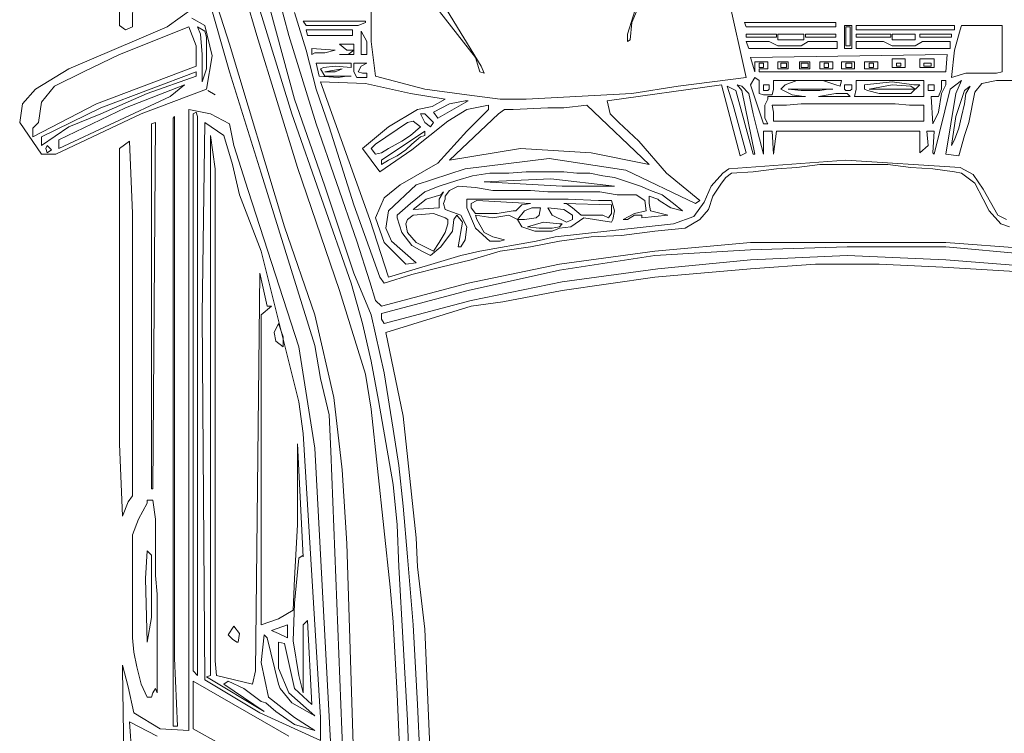
# Model space of a CAD drawing. Units: inches. Extents: x -36302355 to 648, y -221479757 to 75.
# Tile 7 of 37: x 182 to 209, y -484 to -465. Entities that reach past the tile are written whole.
import ezdxf

# ---------------------------------------------------------------- set-up
doc = ezdxf.new("R2010")
doc.units = ezdxf.units.IN
doc.header["$MEASUREMENT"] = 0
doc.layers.add('A-EQPM-VEHC', color=8, linetype='Continuous', lineweight=13)

msp = doc.modelspace()

# ---------------------------------------------------------------- linework, layer by layer
at = {"layer": 'A-EQPM-VEHC'}
for p, q in [((185.107, -459.219), (185.107, -465.157)), ((202.134, -466.571), (201.032, -461.617)), ((185.461, -465.195), (185.5, -462.049)), ((188.842, -465.431), (187.821, -461.932)), ((188.96, -462.6), (189.708, -465.431)), ((191.95, -463.307), (191.95, -465.588)), ((199.736, -463.386), (199.027, -465.078)), ((188.567, -463.583), (189.786, -467.555)), ((198.909, -465.392), (199.46, -463.662)), ((187.467, -464.213), (188.095, -466.415)), ((187.623, -464.172), (188.095, -465.667)), ((187.112, -464.685), (186.405, -465.195)), ((189.865, -467.162), (189.197, -464.723)), ((189.865, -464.802), (190.18, -465.825)), ((193.64, -464.565), (194.78, -466.022)), ((194.938, -466.257), (193.994, -464.723)), ((187.426, -465.157), (187.074, -464.96)), ((190.101, -465.037), (191.792, -465.037)), ((190.18, -465.157), (190.101, -465.037)), ((191.792, -465.037), (191.792, -465.078)), ((185.107, -465.157), (185.265, -465.274)), ((186.995, -465.195), (185.107, -465.943)), ((185.265, -465.274), (185.461, -465.195)), ((186.405, -465.195), (185.579, -465.55)), ((187.191, -465.706), (186.995, -465.195)), ((187.426, -465.313), (187.23, -465.195)), ((187.23, -465.195), (187.309, -465.392)), ((187.623, -465.981), (187.426, -465.157)), ((187.467, -465.471), (187.426, -465.313)), ((191.596, -465.157), (190.18, -465.157)), ((190.18, -465.274), (191.438, -465.274)), ((190.22, -465.431), (190.18, -465.274)), ((191.438, -465.274), (191.438, -465.431)), ((191.792, -465.078), (191.596, -465.157)), ((191.831, -465.588), (191.674, -465.313)), ((191.674, -465.313), (191.674, -465.943)), ((199.027, -465.078), (198.988, -465.55)), ((204.572, -465.078), (202.094, -465.078)), ((202.094, -465.078), (202.134, -465.195)), ((202.134, -465.195), (204.572, -465.195)), ((204.572, -465.195), (204.572, -465.078)), ((205.005, -465.157), (204.808, -465.157)), ((204.808, -465.157), (204.808, -465.785)), ((204.965, -465.195), (204.847, -465.195)), ((204.847, -465.195), (204.847, -465.706)), ((204.965, -465.706), (204.965, -465.195)), ((205.005, -465.785), (205.005, -465.157)), ((207.797, -465.157), (205.123, -465.157)), ((205.123, -465.157), (205.123, -465.274)), ((205.123, -465.274), (207.797, -465.274)), ((207.797, -465.274), (207.797, -465.157)), ((207.953, -465.274), (207.797, -465.825)), ((207.993, -465.157), (207.953, -465.274)), ((209.094, -465.157), (207.993, -465.157)), ((209.094, -466.415), (209.094, -465.157)), ((185.579, -465.55), (183.731, -466.336)), ((187.309, -465.392), (187.349, -465.943)), ((187.467, -466.336), (187.467, -465.471)), ((189.944, -469.01), (188.842, -465.431)), ((189.708, -465.431), (190.455, -467.831)), ((191.438, -465.431), (190.22, -465.431)), ((191.831, -465.943), (191.831, -465.588)), ((191.95, -465.588), (192.068, -466.532)), ((198.909, -465.588), (198.909, -465.392)), ((198.988, -465.55), (198.909, -465.588)), ((202.959, -465.392), (202.134, -465.392)), ((202.134, -465.392), (202.134, -465.471)), ((202.134, -465.471), (202.959, -465.471)), ((202.213, -465.785), (202.134, -465.588)), ((202.134, -465.588), (202.763, -465.588)), ((202.763, -465.588), (202.999, -465.706)), ((202.959, -465.471), (202.959, -465.392)), ((203.707, -465.392), (202.999, -465.392)), ((202.999, -465.392), (202.999, -465.55)), ((202.999, -465.55), (203.707, -465.55)), ((203.628, -465.706), (203.824, -465.588)), ((203.707, -465.55), (203.707, -465.392)), ((204.572, -465.392), (203.747, -465.392)), ((203.747, -465.392), (203.747, -465.471)), ((203.747, -465.471), (204.572, -465.471)), ((203.824, -465.588), (204.612, -465.588)), ((204.572, -465.471), (204.572, -465.392)), ((204.612, -465.588), (204.612, -465.785)), ((206.067, -465.392), (205.123, -465.392)), ((205.123, -465.392), (205.123, -465.471)), ((205.123, -465.471), (206.067, -465.471)), ((205.87, -465.588), (205.123, -465.588)), ((205.123, -465.588), (205.123, -465.785)), ((206.105, -465.706), (205.87, -465.588)), ((206.067, -465.471), (206.067, -465.392)), ((206.735, -465.392), (206.105, -465.392)), ((206.105, -465.392), (206.105, -465.55)), ((206.105, -465.55), (206.735, -465.55)), ((206.735, -465.55), (206.735, -465.392)), ((206.932, -465.588), (206.735, -465.706)), ((207.718, -465.392), (206.853, -465.392)), ((206.853, -465.392), (206.853, -465.471)), ((206.853, -465.471), (207.718, -465.471)), ((207.679, -465.588), (206.932, -465.588)), ((207.679, -465.785), (207.679, -465.588)), ((207.718, -465.471), (207.718, -465.392)), ((187.191, -466.257), (187.191, -465.706)), ((188.095, -465.667), (189.59, -470.623)), ((190.18, -465.825), (190.455, -466.887)), ((190.966, -465.825), (190.337, -465.785)), ((190.337, -465.785), (190.337, -465.943)), ((190.69, -465.903), (190.966, -465.825)), ((191.478, -465.667), (191.085, -465.667)), ((191.085, -465.667), (191.281, -465.825)), ((191.281, -465.825), (191.478, -465.825)), ((191.478, -465.825), (191.32, -465.943)), ((191.478, -465.943), (191.478, -465.667)), ((204.612, -465.785), (202.213, -465.785)), ((202.999, -465.706), (203.628, -465.706)), ((204.808, -465.785), (205.005, -465.785)), ((204.847, -465.706), (204.965, -465.706)), ((205.123, -465.785), (207.679, -465.785)), ((206.735, -465.706), (206.105, -465.706)), ((207.797, -465.825), (207.718, -466.571)), ((185.107, -465.943), (184.124, -466.415)), ((187.349, -465.943), (187.349, -466.69)), ((187.467, -466.887), (187.623, -465.981)), ((190.337, -465.943), (190.416, -465.903)), ((190.416, -465.903), (190.69, -465.903)), ((191.085, -465.943), (191.478, -465.943)), ((191.674, -465.943), (191.831, -465.943)), ((194.78, -466.022), (194.898, -466.415)), ((207.6, -465.943), (202.252, -466.022)), ((202.252, -466.022), (202.369, -466.415)), ((202.369, -466.415), (202.369, -466.139)), ((202.369, -466.139), (202.724, -466.139)), ((202.724, -466.139), (202.724, -466.336)), ((203.275, -466.139), (202.999, -466.139)), ((202.999, -466.139), (202.999, -466.336)), ((203.275, -466.336), (203.275, -466.139)), ((203.864, -466.139), (203.589, -466.139)), ((203.589, -466.139), (203.589, -466.336)), ((203.864, -466.336), (203.864, -466.139)), ((204.14, -466.336), (204.14, -466.139)), ((204.14, -466.139), (204.493, -466.139)), ((204.493, -466.139), (204.493, -466.336)), ((204.729, -466.336), (204.729, -466.139)), ((204.729, -466.139), (205.084, -466.139)), ((205.084, -466.139), (205.084, -466.336)), ((205.712, -466.139), (205.358, -466.139)), ((205.358, -466.139), (205.358, -466.336)), ((205.712, -466.336), (205.712, -466.139)), ((206.46, -466.06), (206.105, -466.06)), ((206.105, -466.06), (206.105, -466.297)), ((206.46, -466.297), (206.46, -466.06)), ((207.246, -466.06), (206.853, -466.06)), ((206.853, -466.06), (206.853, -466.297)), ((207.246, -466.297), (207.246, -466.06)), ((207.56, -466.415), (207.6, -465.943)), ((183.731, -466.336), (182.826, -466.887)), ((184.478, -467.28), (187.191, -466.257)), ((187.349, -466.69), (187.467, -466.336)), ((190.455, -466.178), (190.534, -466.532)), ((191.399, -466.178), (190.455, -466.178)), ((190.573, -466.336), (190.652, -466.297)), ((190.69, -466.532), (190.573, -466.336)), ((190.652, -466.297), (190.966, -466.257)), ((191.162, -466.336), (190.69, -466.415)), ((190.966, -466.257), (191.399, -466.297)), ((190.966, -466.415), (191.162, -466.336)), ((191.399, -466.297), (191.399, -466.178)), ((191.831, -466.178), (191.478, -466.178)), ((191.478, -466.178), (191.478, -466.415)), ((191.596, -466.415), (191.674, -466.257)), ((191.674, -466.257), (191.831, -466.178)), ((195.017, -466.453), (194.938, -466.257)), ((202.487, -466.297), (202.487, -466.178)), ((202.487, -466.178), (202.606, -466.178)), ((202.606, -466.297), (202.487, -466.297)), ((202.724, -466.336), (202.487, -466.336)), ((202.487, -466.336), (202.487, -466.415)), ((202.606, -466.178), (202.606, -466.297)), ((202.999, -466.336), (203.275, -466.336)), ((203.078, -466.297), (203.078, -466.178)), ((203.078, -466.178), (203.235, -466.178)), ((203.235, -466.297), (203.078, -466.297)), ((203.235, -466.178), (203.235, -466.297)), ((203.589, -466.336), (203.864, -466.336)), ((203.628, -466.297), (203.628, -466.178)), ((203.628, -466.178), (203.824, -466.178)), ((203.824, -466.297), (203.628, -466.297)), ((203.824, -466.178), (203.824, -466.297)), ((204.493, -466.336), (204.14, -466.336)), ((204.257, -466.297), (204.257, -466.178)), ((204.257, -466.178), (204.375, -466.178)), ((204.375, -466.297), (204.257, -466.297)), ((204.375, -466.178), (204.375, -466.297)), ((205.084, -466.336), (204.729, -466.336)), ((205.005, -466.178), (204.847, -466.178)), ((204.847, -466.178), (204.847, -466.297)), ((204.847, -466.297), (205.005, -466.297)), ((205.005, -466.297), (205.005, -466.178)), ((205.358, -466.336), (205.712, -466.336)), ((205.477, -466.297), (205.477, -466.178)), ((205.477, -466.178), (205.595, -466.178)), ((205.595, -466.297), (205.477, -466.297)), ((205.595, -466.178), (205.595, -466.297)), ((206.105, -466.297), (206.46, -466.297)), ((206.223, -466.257), (206.223, -466.178)), ((206.223, -466.178), (206.342, -466.178)), ((206.342, -466.257), (206.223, -466.257)), ((206.342, -466.178), (206.342, -466.257)), ((206.853, -466.297), (207.246, -466.297)), ((206.97, -466.257), (206.97, -466.178)), ((206.97, -466.178), (207.167, -466.178)), ((207.167, -466.257), (206.97, -466.257)), ((207.167, -466.178), (207.167, -466.257)), ((184.124, -466.415), (183.338, -466.808)), ((187.191, -466.415), (184.596, -467.397)), ((185.854, -467.004), (187.191, -466.532)), ((187.191, -466.532), (187.191, -466.415)), ((188.095, -466.415), (188.96, -469.166)), ((190.534, -466.532), (191.045, -466.571)), ((190.69, -466.415), (190.966, -466.415)), ((191.399, -466.532), (190.69, -466.532)), ((191.045, -466.571), (191.281, -466.532)), ((191.478, -466.415), (191.555, -466.571)), ((191.555, -466.571), (191.831, -466.571)), ((191.713, -466.453), (191.596, -466.415)), ((191.831, -466.453), (191.713, -466.453)), ((191.831, -466.571), (191.831, -466.453)), ((192.068, -466.532), (193.405, -466.887)), ((194.898, -466.415), (195.017, -466.453)), ((200.285, -466.808), (202.134, -466.571)), ((202.369, -466.571), (202.252, -466.768)), ((202.487, -466.65), (202.369, -466.571)), ((202.487, -466.415), (207.56, -466.415)), ((202.487, -467.004), (202.487, -466.65)), ((204.729, -466.65), (202.882, -466.65)), ((202.882, -466.65), (202.882, -466.887)), ((203.196, -466.768), (203.51, -466.65)), ((204.217, -466.65), (204.572, -466.768)), ((204.689, -466.808), (204.729, -466.65)), ((206.97, -466.65), (205.123, -466.65)), ((205.123, -466.65), (205.123, -466.887)), ((206.97, -467.083), (206.97, -466.65)), ((207.56, -466.65), (207.442, -466.65)), ((207.442, -466.65), (207.442, -466.887)), ((207.56, -466.768), (207.56, -466.65)), ((207.993, -466.65), (207.679, -466.887)), ((207.718, -466.571), (208.111, -466.453)), ((207.835, -467.004), (207.993, -466.65)), ((208.111, -466.453), (208.937, -466.453)), ((208.937, -466.65), (208.544, -466.729)), ((208.937, -466.453), (209.094, -466.415)), ((217.274, -466.65), (208.937, -466.65)), ((182.826, -466.887), (182.473, -467.28)), ((183.338, -466.808), (182.983, -467.24)), ((186.877, -466.768), (185.265, -467.397)), ((185.696, -467.555), (187.467, -466.887)), ((186.484, -467.083), (186.877, -466.768)), ((187.702, -467.043), (187.505, -466.925)), ((190.455, -466.887), (190.809, -467.908)), ((191.792, -466.729), (190.573, -466.69)), ((190.573, -466.69), (191.91, -470.426)), ((193.012, -467.004), (191.792, -466.729)), ((193.405, -466.887), (194.545, -467.043)), ((201.466, -466.768), (198.358, -467.201)), ((199.027, -467.004), (200.285, -466.808)), ((201.976, -468.696), (201.466, -466.768)), ((201.859, -466.925), (201.622, -466.808)), ((201.622, -466.808), (201.78, -467.319)), ((202.331, -468.656), (201.859, -466.925)), ((202.017, -466.808), (201.897, -466.768)), ((201.897, -466.768), (202.017, -466.925)), ((202.213, -467.004), (202.017, -466.808)), ((202.017, -466.925), (202.369, -468.656)), ((202.252, -466.768), (202.606, -467.831)), ((202.763, -466.768), (202.606, -466.768)), ((202.606, -466.768), (202.606, -466.925)), ((202.606, -466.925), (202.724, -466.925)), ((202.724, -466.925), (202.763, -466.887)), ((202.763, -466.887), (202.763, -466.768)), ((202.882, -466.887), (202.841, -467.043)), ((203.078, -466.887), (203.196, -466.768)), ((203.392, -467.043), (203.078, -466.887)), ((203.275, -466.887), (203.628, -466.925)), ((204.493, -466.887), (203.275, -466.887)), ((203.628, -466.925), (204.14, -466.925)), ((204.14, -466.925), (204.375, -466.887)), ((204.572, -466.768), (204.689, -466.808)), ((205.005, -466.768), (204.808, -466.768)), ((204.808, -466.768), (204.808, -466.887)), ((204.808, -466.887), (204.847, -466.925)), ((204.847, -466.925), (204.965, -466.925)), ((204.965, -466.925), (205.005, -466.887)), ((205.005, -466.887), (205.005, -466.768)), ((205.123, -466.887), (205.084, -467.083)), ((206.105, -466.69), (205.358, -466.768)), ((205.358, -466.768), (205.358, -466.887)), ((205.358, -466.887), (205.437, -466.925)), ((205.437, -466.925), (205.751, -467.004)), ((206.105, -466.768), (205.477, -466.887)), ((205.477, -466.887), (206.735, -466.887)), ((206.695, -466.768), (206.105, -466.69)), ((206.616, -466.808), (206.105, -466.768)), ((206.616, -467.004), (206.853, -466.768)), ((206.735, -466.887), (206.616, -466.808)), ((206.853, -466.768), (206.695, -466.768)), ((207.246, -466.768), (207.088, -466.768)), ((207.088, -466.768), (207.088, -466.925)), ((207.088, -466.925), (207.246, -466.925)), ((207.246, -466.925), (207.246, -466.768)), ((207.679, -466.887), (207.246, -468.656)), ((207.442, -466.887), (207.363, -467.083)), ((207.442, -467.004), (207.56, -466.768)), ((208.072, -466.925), (207.835, -467.633)), ((208.228, -466.808), (208.072, -466.925)), ((208.111, -467.004), (208.228, -466.808)), ((208.544, -466.729), (208.348, -466.964)), ((183.455, -468.498), (186.484, -467.083)), ((184.596, -467.555), (185.854, -467.004)), ((190.69, -469.521), (189.865, -467.162)), ((193.954, -467.162), (193.012, -467.004)), ((193.601, -467.359), (193.954, -467.162)), ((193.757, -467.673), (194.584, -467.201)), ((194.505, -467.201), (194.073, -467.28)), ((194.584, -467.201), (194.505, -467.201)), ((194.545, -467.043), (195.449, -467.162)), ((195.449, -467.162), (196.156, -467.162)), ((196.156, -467.162), (199.027, -467.004)), ((198.358, -467.201), (198.437, -467.555)), ((202.331, -467.555), (202.213, -467.004)), ((202.606, -467.043), (202.487, -467.004)), ((202.841, -467.043), (202.606, -467.043)), ((202.645, -467.319), (202.724, -467.162)), ((202.724, -467.162), (202.724, -467.083)), ((202.724, -467.083), (203.747, -467.083)), ((203.707, -467.083), (203.392, -467.043)), ((204.572, -467.004), (204.1, -467.083)), ((204.1, -467.083), (204.965, -467.083)), ((204.886, -467.004), (204.572, -467.004)), ((204.965, -467.083), (204.886, -467.004)), ((205.084, -467.083), (206.97, -467.083)), ((206.616, -467.004), (205.751, -467.004)), ((207.363, -467.083), (207.167, -467.083)), ((207.167, -467.083), (207.207, -467.831)), ((207.363, -467.515), (207.442, -467.004)), ((207.56, -468.656), (207.835, -467.004)), ((208.072, -467.28), (208.111, -467.004)), ((208.348, -466.964), (208.19, -467.791)), ((182.473, -467.28), (182.394, -467.791)), ((182.748, -468.184), (184.478, -467.28)), ((182.983, -467.24), (182.905, -467.791)), ((184.596, -467.397), (182.983, -468.184)), ((185.265, -467.397), (183.455, -468.263)), ((187.584, -467.555), (186.995, -467.436)), ((186.995, -467.436), (186.995, -484.306)), ((192.42, -467.908), (193.208, -467.436)), ((193.208, -467.436), (193.601, -467.359)), ((194.073, -467.28), (193.64, -467.515)), ((194.545, -467.436), (194.033, -467.752)), ((195.135, -467.319), (194.545, -467.436)), ((194.545, -468.027), (195.135, -467.436)), ((195.135, -467.436), (195.135, -467.319)), ((195.567, -467.436), (195.41, -467.555)), ((195.803, -467.436), (195.567, -467.436)), ((196.747, -467.397), (195.803, -467.436)), ((197.179, -467.397), (196.747, -467.397)), ((197.809, -467.319), (197.179, -467.397)), ((199.499, -468.931), (197.809, -467.319)), ((201.78, -467.319), (202.134, -468.617)), ((202.645, -467.673), (202.645, -467.319)), ((203.235, -467.319), (202.841, -467.319)), ((202.841, -467.319), (202.882, -467.515)), ((203.628, -467.28), (203.235, -467.319)), ((206.184, -467.28), (203.628, -467.28)), ((206.577, -467.319), (206.184, -467.28)), ((206.97, -467.319), (206.577, -467.319)), ((206.97, -467.752), (206.97, -467.319)), ((207.993, -467.633), (208.072, -467.28)), ((183.377, -468.656), (185.696, -467.555)), ((183.731, -467.908), (184.596, -467.555)), ((186.602, -467.633), (186.561, -467.673)), ((186.561, -467.673), (186.561, -484.188)), ((186.602, -482.341), (186.602, -467.633)), ((187.191, -467.515), (187.112, -467.555)), ((187.112, -467.555), (187.112, -482.693)), ((187.23, -467.633), (187.191, -467.515)), ((187.23, -482.813), (187.23, -467.633)), ((188.095, -467.831), (187.584, -467.555)), ((189.786, -467.555), (191.399, -472.156)), ((193.089, -467.752), (192.933, -467.791)), ((194.033, -467.752), (193.05, -468.538)), ((193.287, -467.908), (193.089, -467.752)), ((193.405, -467.555), (193.287, -467.555)), ((193.287, -467.555), (193.405, -467.791)), ((193.64, -467.791), (193.405, -467.555)), ((193.64, -467.515), (193.757, -467.673)), ((195.41, -467.555), (194.073, -468.813)), ((198.437, -467.555), (198.674, -467.791)), ((202.448, -468.027), (202.331, -467.555)), ((202.724, -467.831), (202.645, -467.673)), ((202.882, -467.515), (202.882, -467.752)), ((202.882, -467.752), (206.97, -467.752)), ((207.207, -467.831), (207.363, -467.515)), ((207.835, -467.633), (207.718, -468.42)), ((207.914, -467.948), (207.993, -467.633)), ((182.394, -467.791), (182.983, -468.656)), ((182.905, -467.791), (182.748, -467.948)), ((182.748, -467.948), (182.748, -468.184)), ((182.983, -468.42), (183.731, -467.908)), ((185.972, -467.831), (186.089, -467.791)), ((185.972, -477.74), (185.972, -467.831)), ((186.089, -467.791), (186.012, -477.74)), ((187.426, -467.791), (187.349, -473.021)), ((187.939, -468.145), (187.426, -467.791)), ((188.214, -468.42), (188.095, -467.831)), ((190.455, -467.831), (191.555, -471.016)), ((190.809, -467.908), (191.478, -470.031)), ((191.713, -468.498), (192.42, -467.908)), ((192.933, -467.791), (192.068, -468.38)), ((193.012, -468.145), (193.287, -467.908)), ((193.405, -467.791), (193.561, -467.908)), ((193.561, -467.908), (193.64, -467.791)), ((198.674, -467.791), (199.223, -468.301)), ((202.606, -467.831), (202.724, -467.831)), ((207.797, -468.263), (207.914, -467.948)), ((208.19, -467.791), (208.072, -468.145)), ((182.983, -468.184), (182.983, -468.42)), ((183.455, -468.263), (183.455, -468.498)), ((187.702, -469.049), (187.584, -468.145)), ((187.584, -468.145), (187.584, -482.813)), ((188.174, -468.931), (187.939, -468.145)), ((193.405, -468.027), (192.224, -468.813)), ((192.775, -468.301), (193.012, -468.145)), ((193.05, -468.38), (193.287, -468.184)), ((193.287, -468.184), (193.405, -468.145)), ((193.405, -468.145), (193.405, -468.027)), ((193.757, -468.892), (194.545, -468.027)), ((202.606, -468.656), (202.448, -468.027)), ((202.841, -468.027), (202.606, -468.027)), ((202.606, -468.027), (202.606, -468.656)), ((202.882, -468.656), (202.841, -468.027)), ((202.959, -468.027), (202.882, -468.656)), ((206.853, -468.027), (202.959, -468.027)), ((206.853, -468.617), (206.853, -468.027)), ((207.246, -468.027), (207.049, -468.027)), ((207.049, -468.027), (207.088, -468.42)), ((207.207, -468.617), (207.246, -468.027)), ((207.718, -468.42), (207.797, -468.263)), ((208.072, -468.145), (207.914, -468.696)), ((183.141, -468.42), (183.101, -468.498)), ((183.101, -468.498), (183.141, -468.617)), ((183.259, -468.538), (183.141, -468.42)), ((183.141, -468.617), (183.259, -468.538)), ((185.382, -468.301), (185.107, -468.498)), ((185.107, -468.498), (185.107, -476.52)), ((185.461, -470.268), (185.382, -468.301)), ((188.607, -469.638), (188.214, -468.42)), ((192.185, -469.128), (191.713, -468.498)), ((192.068, -468.38), (191.95, -468.498)), ((191.95, -468.498), (192.068, -468.656)), ((193.05, -468.538), (192.185, -469.128)), ((192.224, -468.617), (192.42, -468.498)), ((192.42, -468.498), (192.775, -468.301)), ((192.657, -468.696), (192.892, -468.538)), ((192.892, -468.538), (193.05, -468.38)), ((194.073, -468.813), (196, -468.498)), ((196, -468.498), (197.927, -468.617)), ((199.223, -468.301), (199.971, -469.166)), ((207.088, -468.42), (206.853, -468.617)), ((182.983, -468.656), (183.377, -468.656)), ((192.068, -468.656), (192.224, -468.617)), ((192.224, -468.813), (192.224, -468.931)), ((192.224, -468.931), (192.42, -468.813)), ((192.42, -468.813), (192.657, -468.696)), ((196.786, -468.773), (194.505, -469.049)), ((198.871, -469.089), (196.786, -468.773)), ((197.927, -468.617), (199.499, -468.931)), ((201.662, -469.049), (204.847, -468.813)), ((202.134, -468.617), (201.976, -468.696)), ((202.369, -468.656), (202.331, -468.656)), ((204.847, -468.813), (207.953, -469.01)), ((207.246, -468.656), (207.207, -468.617)), ((207.914, -468.696), (207.56, -468.656)), ((187.702, -482.419), (187.702, -469.049)), ((188.37, -469.757), (188.174, -468.931)), ((191.085, -472.353), (189.944, -469.01)), ((192.736, -469.482), (193.757, -468.892)), ((194.505, -469.049), (193.168, -469.482)), ((200.757, -469.993), (198.871, -469.089)), ((201.504, -469.166), (201.662, -469.049)), ((202.331, -469.128), (202.959, -469.049)), ((202.959, -469.049), (203.51, -469.01)), ((203.51, -469.01), (204.14, -468.931)), ((204.14, -468.931), (205.988, -468.931)), ((205.988, -468.931), (206.616, -469.01)), ((206.616, -469.01), (207.207, -469.049)), ((207.207, -469.049), (207.797, -469.128)), ((207.953, -469.01), (208.307, -469.207)), ((188.96, -469.166), (190.416, -473.846)), ((194.701, -469.245), (194.27, -469.363)), ((195.173, -469.166), (194.701, -469.245)), ((196.825, -469.324), (195.017, -469.403)), ((195.686, -469.166), (195.173, -469.166)), ((196.156, -469.128), (195.686, -469.166)), ((197.179, -469.128), (196.156, -469.128)), ((198.555, -469.521), (196.825, -469.324)), ((197.533, -469.166), (197.179, -469.128)), ((197.886, -469.166), (197.533, -469.166)), ((198.241, -469.245), (197.886, -469.166)), ((198.555, -469.285), (198.241, -469.245)), ((199.264, -469.521), (198.555, -469.285)), ((199.971, -469.166), (200.876, -469.914)), ((201.19, -469.521), (201.504, -469.166)), ((201.466, -469.442), (201.583, -469.285)), ((201.583, -469.285), (201.741, -469.166)), ((201.741, -469.166), (202.331, -469.128)), ((207.797, -469.128), (207.993, -469.166)), ((207.993, -469.166), (208.348, -469.442)), ((208.307, -469.207), (208.583, -469.6)), ((191.478, -471.881), (190.69, -469.521)), ((192.303, -469.835), (192.736, -469.482)), ((193.168, -469.482), (192.42, -470.189)), ((193.798, -469.521), (193.405, -469.679)), ((194.27, -469.363), (193.798, -469.521)), ((194.073, -469.638), (194.308, -469.521)), ((194.308, -469.521), (194.78, -469.561)), ((194.78, -469.561), (195.252, -469.638)), ((195.017, -469.403), (197.14, -469.521)), ((197.14, -469.521), (198.555, -469.521)), ((199.539, -469.638), (199.264, -469.521)), ((200.994, -469.954), (201.19, -469.521)), ((201.229, -469.796), (201.466, -469.442)), ((208.348, -469.442), (208.583, -469.875)), ((208.583, -469.6), (208.976, -470.307)), ((188.96, -471.291), (188.37, -469.757)), ((189.983, -473.886), (188.607, -469.638)), ((192.068, -470.386), (192.303, -469.835)), ((193.405, -469.679), (193.012, -469.993)), ((193.443, -469.875), (193.089, -470.151)), ((193.836, -469.757), (193.443, -469.875)), ((193.798, -469.875), (193.915, -469.679)), ((193.798, -470.11), (193.798, -469.875)), ((193.915, -469.679), (193.836, -469.757)), ((193.915, -469.993), (193.954, -469.875)), ((193.954, -469.796), (194.073, -469.638)), ((193.954, -469.875), (193.954, -469.796)), ((197.297, -469.875), (194.545, -469.875)), ((194.545, -469.875), (194.545, -470.11)), ((195.252, -469.638), (196.275, -469.638)), ((196.275, -469.638), (196.747, -469.679)), ((196.747, -469.679), (198.162, -469.679)), ((198.123, -469.914), (197.297, -469.875)), ((198.162, -469.679), (198.634, -469.757)), ((198.634, -469.757), (199.146, -469.757)), ((199.146, -469.757), (199.381, -469.914)), ((199.499, -469.993), (199.499, -469.796)), ((199.499, -469.796), (199.736, -469.875)), ((199.853, -469.757), (199.539, -469.638)), ((199.736, -469.875), (199.774, -469.914)), ((200.167, -469.993), (199.853, -469.757)), ((201.111, -470.151), (201.229, -469.796)), ((208.583, -469.875), (208.741, -470.189)), ((191.478, -470.031), (192.185, -471.998)), ((193.012, -469.993), (192.657, -470.307)), ((193.089, -470.151), (193.798, -470.11)), ((193.954, -470.151), (193.915, -469.993)), ((194.387, -470.307), (193.954, -470.151)), ((194.545, -470.11), (194.78, -470.661)), ((194.819, -469.914), (194.663, -469.993)), ((194.663, -469.993), (194.663, -470.11)), ((194.663, -470.11), (194.78, -470.268)), ((196.275, -469.993), (194.819, -469.914)), ((195.882, -470.189), (196.039, -470.031)), ((196.039, -470.031), (196.275, -469.993)), ((196.314, -470.11), (196.117, -470.189)), ((196.551, -470.11), (196.314, -470.11)), ((196.511, -470.307), (196.551, -470.11)), ((197.179, -470.151), (196.747, -470.11)), ((196.747, -470.11), (196.865, -470.307)), ((198.477, -470.031), (197.179, -469.993)), ((197.179, -469.993), (197.258, -469.993)), ((197.416, -470.307), (197.179, -470.151)), ((197.258, -469.993), (197.416, -470.11)), ((197.416, -470.11), (197.651, -470.307)), ((198.477, -469.914), (198.123, -469.914)), ((198.555, -470.189), (198.477, -469.914)), ((198.477, -470.268), (198.477, -470.031)), ((199.381, -469.914), (199.42, -470.189)), ((199.539, -470.189), (199.499, -469.993)), ((199.774, -469.914), (200.088, -470.11)), ((200.088, -470.11), (200.404, -470.189)), ((200.404, -470.189), (200.167, -469.993)), ((200.718, -470.347), (200.994, -469.954)), ((200.876, -469.914), (200.757, -469.993)), ((200.876, -470.426), (201.111, -470.151)), ((185.461, -477.936), (185.461, -470.268)), ((191.91, -470.426), (192.42, -471.998)), ((192.303, -471.054), (192.068, -470.386)), ((192.42, -470.189), (192.343, -470.661)), ((192.657, -470.307), (192.657, -470.386)), ((192.657, -470.386), (192.775, -470.779)), ((192.933, -470.426), (192.892, -470.544)), ((193.089, -470.307), (192.933, -470.426)), ((193.64, -470.268), (193.089, -470.307)), ((193.954, -470.386), (193.64, -470.268)), ((194.033, -470.426), (193.954, -470.386)), ((194.033, -470.544), (194.033, -470.426)), ((194.152, -470.74), (194.191, -470.426)), ((194.191, -470.426), (194.27, -470.307)), ((194.27, -470.307), (194.426, -470.503)), ((194.545, -470.623), (194.387, -470.307)), ((194.78, -470.268), (195.37, -470.268)), ((194.819, -470.426), (194.78, -470.307)), ((194.78, -470.307), (195.252, -470.386)), ((195.017, -470.779), (194.819, -470.426)), ((195.252, -470.386), (195.686, -470.307)), ((195.37, -470.268), (195.803, -470.189)), ((195.686, -470.307), (195.921, -470.426)), ((195.803, -470.189), (195.882, -470.189)), ((196.117, -470.189), (195.921, -470.426)), ((195.921, -470.426), (196.039, -470.623)), ((195.921, -470.426), (196.117, -470.426)), ((196.117, -470.426), (196.432, -470.386)), ((196.432, -470.386), (196.511, -470.307)), ((196.865, -470.307), (197.258, -470.503)), ((197.258, -470.503), (197.416, -470.426)), ((197.376, -470.623), (197.73, -470.386)), ((197.416, -470.426), (197.416, -470.307)), ((197.651, -470.307), (198.241, -470.307)), ((197.73, -470.386), (198.477, -470.503)), ((198.241, -470.307), (198.399, -470.386)), ((198.399, -470.386), (198.477, -470.268)), ((198.477, -470.503), (198.516, -470.426)), ((198.516, -470.426), (198.555, -470.189)), ((199.106, -470.268), (198.792, -470.426)), ((198.792, -470.426), (198.909, -470.426)), ((198.909, -470.426), (199.106, -470.307)), ((199.42, -470.189), (199.106, -470.268)), ((199.106, -470.307), (199.302, -470.307)), ((199.302, -470.307), (199.302, -470.386)), ((199.302, -470.386), (200.011, -470.307)), ((200.011, -470.307), (199.539, -470.189)), ((200.167, -470.544), (200.718, -470.347)), ((200.483, -470.661), (200.876, -470.426)), ((208.741, -470.189), (209.055, -470.544)), ((208.976, -470.307), (209.213, -470.426)), ((189.59, -470.623), (190.416, -473.021)), ((192.343, -470.661), (192.499, -471.016)), ((192.892, -470.544), (192.933, -470.779)), ((193.954, -470.779), (194.033, -470.544)), ((194.426, -470.503), (194.308, -471.172)), ((194.505, -470.975), (194.545, -470.623)), ((194.78, -470.661), (195.173, -471.016)), ((196.039, -470.623), (196.393, -470.74)), ((196.628, -470.503), (196.196, -470.623)), ((196.196, -470.623), (196.511, -470.661)), ((196.511, -470.661), (196.865, -470.661)), ((197.061, -470.544), (196.628, -470.503)), ((196.865, -470.661), (197.061, -470.623)), ((196.865, -470.74), (197.061, -470.661)), ((196.944, -470.896), (200.167, -470.544)), ((197.061, -470.623), (197.14, -470.544)), ((197.14, -470.544), (197.061, -470.544)), ((197.061, -470.661), (197.376, -470.623)), ((199.657, -470.74), (200.483, -470.661)), ((209.055, -470.544), (209.29, -470.623)), ((192.775, -470.779), (193.05, -471.133)), ((192.933, -470.779), (193.168, -471.054)), ((193.798, -471.054), (193.954, -470.779)), ((193.836, -471.172), (194.152, -470.74)), ((195.252, -470.896), (195.017, -470.779)), ((195.567, -470.975), (195.252, -470.896)), ((196.393, -470.74), (196.865, -470.74)), ((196.432, -471.016), (196.944, -470.896)), ((197.061, -471.016), (197.927, -470.896)), ((197.927, -470.896), (198.751, -470.858)), ((198.751, -470.858), (199.657, -470.74)), ((191.555, -471.016), (191.91, -472.116)), ((192.892, -471.644), (192.303, -471.054)), ((192.499, -471.016), (193.168, -471.605)), ((193.05, -471.133), (193.326, -471.291)), ((193.168, -471.054), (193.64, -471.291)), ((193.561, -471.409), (193.836, -471.172)), ((193.64, -471.291), (193.798, -471.054)), ((194.308, -471.172), (194.387, -471.172)), ((194.387, -471.172), (194.505, -470.975)), ((194.898, -471.291), (196.432, -471.016)), ((195.173, -471.016), (195.449, -471.016)), ((195.449, -471.016), (195.567, -470.975)), ((195.449, -471.291), (196.275, -471.172)), ((196.275, -471.172), (197.061, -471.016)), ((199.657, -471.291), (202.252, -471.054)), ((202.252, -471.054), (207.56, -471.054)), ((204.886, -471.172), (202.252, -471.251)), ((207.56, -471.172), (204.886, -471.172)), ((207.56, -471.054), (210.195, -471.251)), ((210.155, -471.409), (207.56, -471.172)), ((189.983, -475.38), (188.96, -471.291)), ((192.42, -471.998), (194.387, -471.409)), ((193.326, -471.291), (193.561, -471.409)), ((194.387, -471.409), (194.898, -471.291)), ((194.663, -471.526), (195.449, -471.291)), ((197.061, -471.644), (199.657, -471.291)), ((199.657, -471.409), (197.061, -471.802)), ((202.252, -471.251), (199.657, -471.409)), ((202.252, -471.526), (204.886, -471.409)), ((204.886, -471.409), (207.56, -471.526)), ((193.168, -471.605), (192.892, -471.644)), ((193.05, -471.919), (193.836, -471.723)), ((193.836, -471.723), (194.663, -471.526)), ((194.584, -472.156), (197.061, -471.644)), ((197.14, -472.116), (199.736, -471.763)), ((202.252, -471.763), (199.657, -471.998)), ((199.736, -471.763), (202.252, -471.526)), ((204.021, -471.644), (202.252, -471.763)), ((205.751, -471.644), (204.021, -471.644)), ((207.483, -471.723), (205.751, -471.644)), ((210.078, -471.881), (207.483, -471.723)), ((207.56, -471.526), (210.155, -471.723)), ((188.921, -471.881), (188.804, -482.693)), ((189.118, -472.784), (188.921, -471.881)), ((191.95, -473.021), (191.478, -471.881)), ((192.185, -471.998), (192.303, -472.156)), ((192.303, -472.156), (193.05, -471.919)), ((197.061, -471.802), (194.584, -472.353)), ((199.657, -471.998), (197.14, -472.353)), ((191.399, -472.156), (191.713, -473.256)), ((191.91, -472.116), (192.068, -472.628)), ((192.224, -472.784), (194.584, -472.156)), ((194.663, -472.628), (197.14, -472.116)), ((191.792, -474.632), (191.085, -472.353)), ((194.584, -472.353), (192.224, -472.981)), ((197.14, -472.353), (195.528, -472.667)), ((188.96, -473.021), (189.236, -472.784)), ((189.236, -472.784), (189.118, -472.784)), ((192.068, -472.628), (192.224, -472.784)), ((192.303, -473.256), (194.663, -472.628)), ((194.663, -472.784), (192.343, -473.493)), ((195.528, -472.667), (194.663, -472.784)), ((187.349, -473.021), (187.426, -482.93)), ((188.96, -481.435), (188.96, -473.021)), ((190.416, -473.021), (190.927, -475.262)), ((192.303, -474.594), (191.95, -473.021)), ((192.224, -472.981), (192.224, -473.139)), ((189.432, -473.256), (189.314, -473.493)), ((189.551, -473.611), (189.432, -473.256)), ((191.713, -473.256), (191.95, -474.279)), ((192.224, -473.139), (192.303, -473.256)), ((189.314, -473.493), (189.355, -473.728)), ((189.551, -473.886), (189.551, -473.611)), ((192.343, -473.493), (192.815, -475.773)), ((189.355, -473.728), (189.551, -473.886)), ((190.416, -476.638), (189.983, -473.886)), ((190.416, -473.846), (190.573, -474.751)), ((191.95, -474.279), (192.146, -475.341)), ((191.95, -475.576), (191.792, -474.632)), ((192.54, -476.127), (192.303, -474.594)), ((190.573, -474.751), (190.809, -475.734)), ((190.101, -476.245), (189.983, -475.38)), ((190.927, -475.262), (191.162, -477.227)), ((192.146, -475.341), (192.54, -477.622)), ((190.809, -475.734), (190.848, -476.717)), ((192.461, -480.414), (191.95, -475.576)), ((192.815, -475.773), (193.168, -479.077)), ((190.573, -483.953), (190.101, -476.245)), ((192.696, -477.11), (192.54, -476.127)), ((185.107, -476.52), (185.186, -478.487)), ((190.101, -479.587), (189.944, -476.52)), ((189.944, -476.52), (189.944, -478.722)), ((190.848, -484.778), (190.416, -476.638)), ((190.848, -476.717), (191.202, -485.643)), ((192.815, -478.212), (192.696, -477.11)), ((191.162, -477.227), (191.281, -479.233)), ((192.54, -477.622), (192.657, -478.722)), ((186.012, -477.74), (185.972, -477.74)), ((185.186, -478.487), (185.343, -478.094)), ((185.343, -478.094), (185.461, -477.936)), ((185.854, -478.133), (185.619, -478.565)), ((186.012, -478.054), (185.854, -478.054)), ((185.854, -478.054), (185.854, -478.133)), ((186.089, -478.565), (186.012, -478.054)), ((192.933, -479.587), (192.815, -478.212)), ((185.619, -478.565), (185.461, -478.998)), ((186.089, -480.098), (186.089, -478.565)), ((189.944, -478.722), (189.865, -480.177)), ((192.657, -478.722), (192.696, -479.863)), ((185.461, -478.998), (185.461, -481.79)), ((191.281, -479.233), (191.478, -485.211)), ((193.168, -479.077), (193.208, -479.863)), ((185.854, -479.43), (185.815, -480.177)), ((185.972, -479.549), (185.854, -479.43)), ((185.972, -481.239), (185.972, -479.549)), ((189.865, -480.846), (189.983, -479.628)), ((189.983, -479.628), (190.101, -479.549)), ((190.101, -479.549), (190.101, -479.587)), ((193.089, -481.435), (192.933, -479.587)), ((192.696, -479.863), (192.933, -484.03)), ((193.208, -479.863), (193.405, -481.554)), ((185.815, -480.177), (185.854, -481.907)), ((186.13, -480.61), (186.089, -480.098)), ((189.865, -480.177), (189.825, -481.042)), ((192.54, -481.358), (192.461, -480.414)), ((186.13, -483.285), (186.13, -480.61)), ((189.825, -481.869), (189.865, -480.846)), ((189.825, -481.042), (189.432, -481.279)), ((185.854, -481.907), (185.972, -481.239)), ((189.432, -481.279), (188.96, -481.435)), ((190.22, -481.318), (190.101, -481.435)), ((190.337, -483.599), (190.22, -481.318)), ((192.657, -483.323), (192.54, -481.358)), ((188.214, -481.475), (188.056, -481.711)), ((188.37, -481.672), (188.214, -481.475)), ((189.669, -481.435), (189.236, -481.593)), ((189.236, -481.593), (189.432, -481.672)), ((189.669, -481.79), (189.669, -481.435)), ((190.101, -481.435), (190.101, -483.285)), ((193.208, -483.599), (193.089, -481.435)), ((193.405, -481.554), (194.426, -505.069)), ((185.461, -481.79), (185.5, -482.183)), ((188.056, -481.711), (188.174, -481.828)), ((188.174, -481.828), (188.292, -481.907)), ((188.292, -481.907), (188.332, -481.907)), ((188.332, -481.907), (188.37, -481.672)), ((188.96, -482.458), (189.039, -481.711)), ((189.039, -481.711), (189.118, -481.79)), ((189.118, -481.79), (189.432, -483.048)), ((189.432, -481.672), (189.669, -481.79)), ((189.432, -482.616), (189.432, -481.907)), ((189.432, -481.907), (189.59, -481.947)), ((189.983, -482.813), (189.825, -481.869)), ((185.5, -482.183), (185.579, -482.576)), ((189.59, -481.947), (189.865, -483.165)), ((186.681, -484.188), (186.602, -482.341)), ((187.742, -482.813), (187.702, -482.419)), ((189.157, -483.402), (188.96, -482.458)), ((185.343, -483.127), (185.186, -482.537)), ((185.186, -482.537), (185.186, -482.655)), ((185.186, -482.655), (185.461, -499.721)), ((185.579, -482.576), (185.696, -483.048)), ((187.112, -482.693), (187.23, -482.813)), ((188.804, -482.693), (188.725, -483.048)), ((189.708, -483.285), (189.432, -482.616)), ((189.708, -484.464), (187.112, -482.969)), ((187.112, -482.969), (187.112, -484.267)), ((187.426, -482.93), (188.921, -483.834)), ((187.584, -482.813), (187.467, -482.851)), ((187.467, -482.851), (189.039, -483.795)), ((188.725, -483.048), (187.742, -482.813)), ((187.939, -483.048), (188.056, -482.969)), ((188.056, -482.969), (188.488, -483.165)), ((190.101, -483.285), (189.983, -482.813)), ((185.5, -483.834), (185.343, -483.127)), ((185.696, -483.048), (185.854, -483.402)), ((186.012, -483.285), (186.089, -483.165)), ((186.089, -483.165), (186.13, -483.285)), ((189.039, -483.795), (187.939, -483.048)), ((188.488, -483.165), (188.96, -483.52)), ((189.432, -483.048), (189.472, -483.165)), ((189.472, -483.165), (189.786, -483.56)), ((189.865, -483.165), (190.337, -483.599)), ((185.854, -483.402), (185.972, -483.402)), ((185.972, -483.402), (186.012, -483.285)), ((188.96, -483.52), (189.079, -483.56)), ((189.865, -483.953), (189.157, -483.402)), ((190.416, -483.913), (189.708, -483.285)), ((193.522, -504.518), (192.657, -483.323)), ((189.079, -483.56), (189.355, -483.795)), ((189.355, -483.795), (189.865, -484.15)), ((189.786, -483.56), (190.416, -483.913)), ((194.073, -503.929), (193.208, -483.599)), ((185.579, -486.941), (185.382, -484.071)), ((185.382, -484.071), (186.13, -484.464)), ((186.209, -484.267), (185.5, -483.834)), ((188.921, -483.834), (190.573, -484.581)), ((190.416, -484.306), (189.865, -483.953)), ((190.573, -484.581), (190.573, -483.953)), ((192.933, -484.03), (193.836, -505.148)), ((186.995, -484.306), (186.209, -484.267)), ((186.561, -484.188), (186.681, -484.188)), ((187.112, -484.267), (187.821, -484.66)), ((189.865, -484.15), (190.416, -484.306))]:
    msp.add_line(p, q, dxfattribs=at)

doc.saveas('drawing.dxf')
